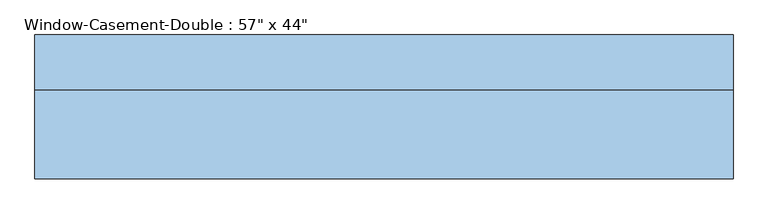
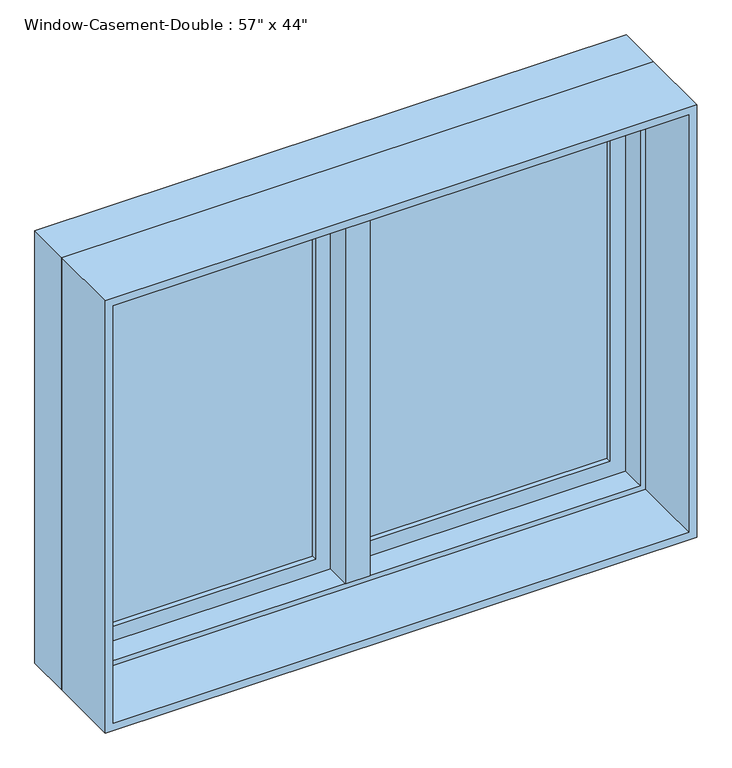
"""IFC4 building model written with IfcOpenShell, lengths in millimetres: window geometry."""

from ifc_helpers import new_model, si_unit, frame, origin, place, context, project, spatial, polyline, outline, extrude, faceted_brep, source, transform, mapped, element, save


def window_2333f571(model_context):
    return source(origin(), model_context, "Body", "SolidModel", [
        faceted_brep([(9.525, 158.75, 2019.3), (-9.525, 158.75, 2019.3), (-9.525, 107.95, 2019.3), (9.525, 107.95, 2019.3), (9.525, 158.75, 927.1), (9.525, 107.95, 927.1), (-9.525, 107.95, 927.1), (-9.525, 158.75, 927.1), (-9.525, 107.95, 946.15), (-9.525, 107.95, 2000.25), (-30.1625, 107.95, 946.15), (-30.1625, 107.95, 2000.25), (-30.1625, 44.45, 946.15), (-30.1625, 44.45, 2000.25), (30.1625, 44.45, 946.15), (30.1625, 44.45, 2000.25), (30.1625, 107.95, 946.15), (30.1625, 107.95, 2000.25), (9.525, 107.95, 946.15), (9.525, 107.95, 2000.25)], [[[0, 1, 2, 3]], [[4, 5, 6, 7]], [[1, 0, 4, 7]], [[2, 1, 7, 6, 8, 9]], [[9, 8, 10, 11]], [[11, 10, 12, 13]], [[13, 12, 14, 15]], [[15, 14, 16, 17]], [[17, 16, 18, 19]], [[0, 3, 19, 18, 5, 4]], [[18, 8, 6, 5]], [[9, 19, 3, 2]], [[8, 18, 16, 14, 12, 10]], [[19, 9, 11, 13, 15, 17]]]),
        extrude(outline(polyline([(-66.675, 139.7), (-66.675, 133.35), (-654.05, 133.35), (-654.05, 139.7), (-66.675, 139.7)])), frame((0.0, 0.0, 984.25), z_axis=(0.0, 0.0, 1.0), x_axis=(1.0, 0.0, 0.0)), (0.0, 0.0, 1.0), 977.9),
        extrude(outline(polyline([(-654.05, 120.65), (-654.05, 127.0), (-66.675, 127.0), (-66.675, 120.65), (-654.05, 120.65)])), frame((0.0, 0.0, 984.25), z_axis=(0.0, 0.0, 1.0), x_axis=(1.0, 0.0, 0.0)), (0.0, 0.0, 1.0), 977.9),
        extrude(outline(polyline([(654.05, 139.7), (654.05, 133.35), (66.675, 133.35), (66.675, 139.7), (654.05, 139.7)])), frame((0.0, 0.0, 984.25), z_axis=(0.0, 0.0, 1.0), x_axis=(1.0, 0.0, 0.0)), (0.0, 0.0, 1.0), 977.9),
        extrude(outline(polyline([(66.675, 120.65), (66.675, 127.0), (654.05, 127.0), (654.05, 120.65), (66.675, 120.65)])), frame((0.0, 0.0, 984.25), z_axis=(0.0, 0.0, 1.0), x_axis=(1.0, 0.0, 0.0)), (0.0, 0.0, 1.0), 977.9),
        extrude(outline(polyline([(2019.3, -711.2), (927.1, -711.2), (927.1, -9.525), (2019.3, -9.525), (2019.3, -711.2)]), holes=[polyline([(1962.15, -66.675), (984.25, -66.675), (984.25, -654.05), (1962.15, -654.05), (1962.15, -66.675)])]), frame((0.0, 107.95, 0.0), z_axis=(0.0, 1.0, 0.0), x_axis=(0.0, 0.0, 1.0)), (0.0, 0.0, 1.0), 44.45),
        extrude(outline(polyline([(927.1, 711.2), (2019.3, 711.2), (2019.3, 9.525), (927.1, 9.525), (927.1, 711.2)]), holes=[polyline([(984.25, 66.675), (1962.15, 66.675), (1962.15, 654.05), (984.25, 654.05), (984.25, 66.675)])]), frame((0.0, 107.95, 0.0), z_axis=(0.0, 1.0, 0.0), x_axis=(0.0, 0.0, 1.0)), (0.0, 0.0, 1.0), 44.45),
        extrude(outline(polyline([(2032.0, -723.9), (914.4, -723.9), (914.4, 723.9), (2032.0, 723.9), (2032.0, -723.9)]), holes=[polyline([(2012.95, 704.85), (933.45, 704.85), (933.45, -704.85), (2012.95, -704.85), (2012.95, 704.85)])]), frame((0.0, -139.7, 0.0), z_axis=(0.0, 1.0, 0.0), x_axis=(0.0, 0.0, 1.0)), (0.0, 0.0, 1.0), 184.15),
        faceted_brep([(692.15, 107.95, 2000.25), (692.15, 44.45, 2000.25), (-692.15, 44.45, 2000.25), (-692.15, 107.95, 2000.25), (711.2, 158.75, 2019.3), (711.2, 107.95, 2019.3), (-711.2, 107.95, 2019.3), (-711.2, 158.75, 2019.3), (723.9, 44.45, 2032.0), (723.9, 158.75, 2032.0), (-723.9, 158.75, 2032.0), (-723.9, 44.45, 2032.0), (-692.15, 44.45, 946.15), (-692.15, 107.95, 946.15), (-711.2, 107.95, 927.1), (-711.2, 158.75, 927.1), (-723.9, 158.75, 914.4), (-723.9, 44.45, 914.4), (692.15, 44.45, 946.15), (692.15, 107.95, 946.15), (711.2, 107.95, 927.1), (711.2, 158.75, 927.1), (723.9, 158.75, 914.4), (723.9, 44.45, 914.4)], [[[0, 1, 2, 3]], [[4, 5, 6, 7]], [[8, 9, 10, 11]], [[3, 2, 12, 13]], [[7, 6, 14, 15]], [[11, 10, 16, 17]], [[13, 12, 18, 19]], [[15, 14, 20, 21]], [[17, 16, 22, 23]], [[11, 17, 23, 8], [1, 18, 12, 2]], [[19, 18, 1, 0]], [[5, 20, 14, 6], [3, 13, 19, 0]], [[21, 20, 5, 4]], [[23, 22, 9, 8]], [[9, 22, 16, 10], [7, 15, 21, 4]]]),
    ])


if __name__ == "__main__":
    model = new_model("IFC4")
    model_context = context("Model", 3, world=origin())
    ifc_project = project(units=[si_unit("LENGTHUNIT", "METRE", prefix="MILLI")], contexts=[model_context])
    site = spatial("IfcSite", under=ifc_project)
    building = spatial("IfcBuilding", under=site)
    placement = place(None, origin())
    window_shape = window_2333f571(model_context)
    element("IfcWindow", 1, ObjectType="Window-Casement-Double : 57\" x 44\"", at=placement, inside=building, context=model_context, shape_type="MappedRepresentation", body=[
        mapped(window_shape, transform((0.0, 0.0, 0.0), x_axis=(1.0, 0.0, 0.0), y_axis=(0.0, 1.0, 0.0), z_axis=(0.0, 0.0, 1.0))),
    ])
    save(model, "model.ifc")

# Revit data of these elements
# Type "Window-Casement-Double : 57\" x 44\""
#   Type Mark = "17"
#   Fire Rating = "0.5h"
#   Assembly Code = "B2020100"
#   Analytic Construction = "Double glazing - domestic"
#   Frame Extension [instance default] = 0.25"
#   Window Inset [instance default] = 0"
#   Wall Thickness [instance default] = 6"
#   Interior Wall Closure [instance default] = 2.25"
#   Half Width = 28.5"
#   Visual Light Transmittance = 0.81
#   Thermal Resistance (R) = 1.8146 (h·ft²·°F)/BTU
#   Solar Heat Gain Coefficient = 0.76
#   Rough Width = 57.5"
#   Rough Height = 44.5"
#   Height = 44"
#   Heat Transfer Coefficient (U) = 0.5511 BTU/(h·ft²·°F)
#   Exterior Wall Closure [instance default] = 1.25"
#   Extension Jamb [instance default] = 2.25"
#   Default Sill Height = 36"
#   Width = 57"
#   Define Thermal Properties by = 0
#   Muntin Visibility = yes
#   Interior Trim Visibility [instance default] = yes
#   Exterior Trim Visibility [instance default] = yes
#   Extension Jamb Visibility [instance default] = yes
#   Interior Trim Material = Wood - Stained
#   Muntin Pattern = Muntin Pattern_2x2 : Muntin Pattern_2x2
#   Interior Trim = Trim-Window-Interior-Flat : Picture Frame
#   Interior Frame Material = Wood - Stained
#   Glass Panel Material = Glass
#   Exterior Trim Material = Clad - White
#   Exterior Trim = Trim-Window-Exterior-Flat : with Sill
#   Exterior Frame Material = Clad - White
#   Wall Closure = (empty or 0)
# Element 1 (IfcWindow, "Window-Casement-Double : 57\" x 44\"")
#   Wall Thickness = 11"
#   Extension Jamb = 7.25"
#   Materials on its faces: "Wood - Stained", "Glass", "Clad - White"
# Materials
#   "Wood - Stained": class "Wood", colour RGB 224 178 126, transparency 0, Cost = 0
#   "Glass": class "Glass", colour RGB 0 128 192, transparency 0.75, Description = "Soda Lime Glass", Cost = 0
#   "Clad - White": class "Wood", colour RGB 242 242 238, transparency 0, Cost = 0
